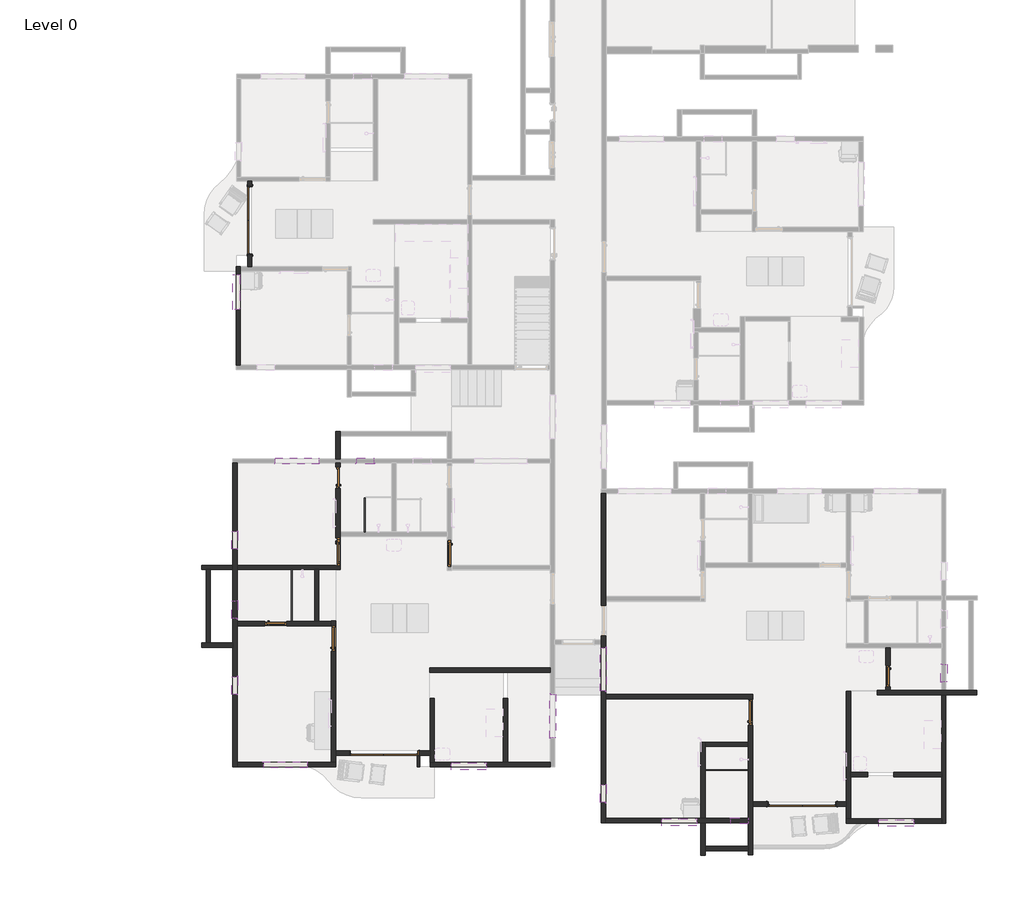
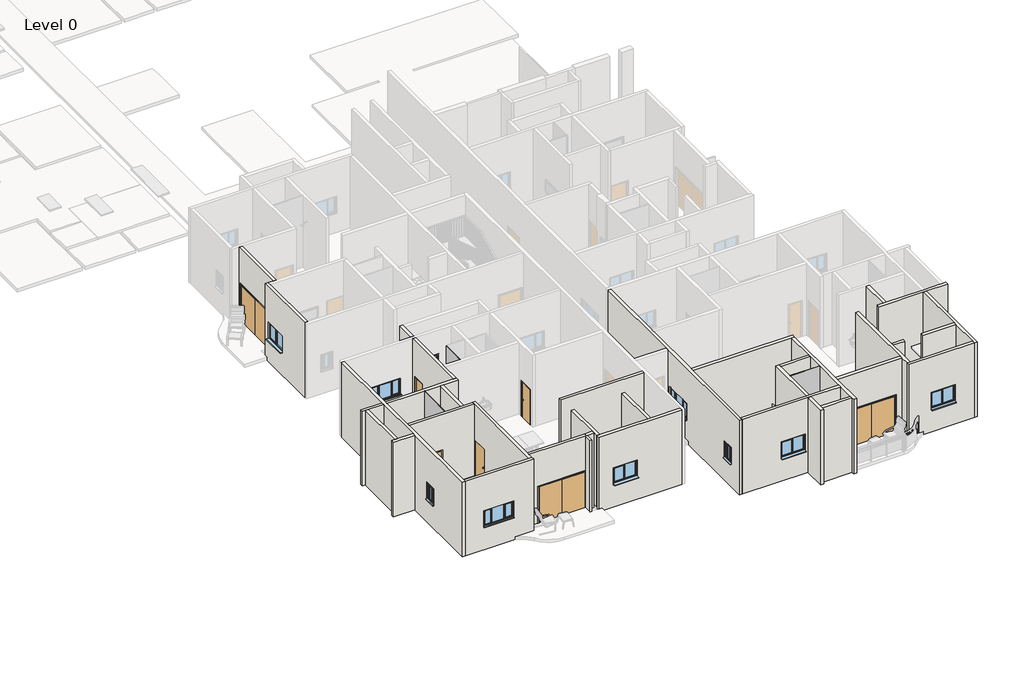
# One storey, part 1 of 14: 33 walls, 15 windows, 11 doors, 3 plates.
# Revit data of these elements (continued)
# Type "Windows_Tpl_Variable_Casement : 5'" (continued)
#   Visual Light Transmittance = 0.9
#   Solar Heat Gain Coefficient = 0.78
#   Rough Width = 1524 mm
#   Rough Height = 910 mm
#   Height = 910 mm
#   Width = 1524 mm
#   Heat Transfer Coefficient (U) = 3.6886 W/(m²·K)
#   Glazing Thickness = 24 mm
#   FrameOffset - External = 50 mm
#   Frame Depth = 65 mm
#   Default Head Height = 2110 mm
#   Cill Depth = 87.5 mm
#   Cavity Closer Width = 50 mm
#   Cavity Closer Offset from Ext = 102.5 mm
#   Cavity Closer Depth = 85 mm
#   Casement Width = 450 mm
#   Vis - Cavity Closers = yes
#   Define Thermal Properties by = 1
#   Material Trim = Window Frame
#   Material Glass = Glass
#   Material Frame = Window Frame
#   Wall Closure = (empty or 0)
# Elements 1, 2, 3 (IfcDoor, "Doors_Concept_IntDbl : 8'")
#   Phase Created = New Construction
#   Materials on its faces: "Glass", "Glass, Clear Glazing"
# Elements 4, 5, 6, 7, 8 (IfcDoor, "Doors_ExtSgl_Flush : D2")
#   Phase Created = New Construction
#   Materials on its faces: "Door - Handle", "Door - Frame/Mullion", "Door - Panel"
# Elements 9, 10, 11 (IfcDoor, "Doors_ExtSgl_Flush : D3")
#   Phase Created = New Construction
#   Materials on its faces: "Door - Handle", "Door - Frame/Mullion", "Door - Panel"
# Elements 12, 13, 14 (IfcPlate, "System Panel : Glazed")
#   Phase Created = New Construction
#   Materials on its faces: "Glass"
# Elements 15, 16, 17, 18, 19, 20, 21, 22, 23, 24, 25, 26, 27, 28, 29, 30, 31, 32, 33, 34, 35, 36, 37, 38, 39, 40, 41, 42, 43, 44, 45, 46 (IfcWall, "W1")
#   Top Offset = 0 mm
#   Base Offset = 0 mm
#   wall height = 4000 mm
#   Phase Created = New Construction
#   Base Constraint = Level 0
#   Top Constraint = Level 1
#   Materials on its faces: "Brick, Common"
# Element 47 (IfcWall, "W9")
#   Top Offset = 0 mm
#   Base Offset = 0 mm
#   wall height = 4000 mm
#   Phase Created = New Construction
#   Base Constraint = Level 0
#   Top Constraint = Level 1
#   Materials on its faces: "Brick, Common"
# Element 48 (IfcWindow, "Windows_Concept_Plain_Dbl : 4'")
#   Mark = "1"
#   Phase Created = New Construction
#   Materials on its faces: "Window Frame", "Glass"
# Element 49 (IfcWindow, "Windows_Concept_Plain_Dbl : 4'")
#   Mark = "12"
#   Phase Created = New Construction
#   Materials on its faces: "Window Frame", "Glass"
# Element 50 (IfcWindow, "Windows_Concept_Plain_Dbl : 4'")
#   Mark = "19"
#   Phase Created = New Construction
#   Materials on its faces: "Window Frame", "Glass"
# Element 51 (IfcWindow, "Windows_Concept_Plain_Dbl : 4'")
#   Mark = "65"
#   Phase Created = New Construction
#   Materials on its faces: "Window Frame", "Glass"
# Element 52 (IfcWindow, "Windows_Sgl_Plain : 2'")
#   Mark = "4"
#   Phase Created = New Construction
#   Materials on its faces: "Window Frame", "Glass"
# Element 53 (IfcWindow, "Windows_Sgl_Plain : 2'")
#   Mark = "5"
#   Phase Created = New Construction
#   Materials on its faces: "Window Frame", "Glass"
# Element 54 (IfcWindow, "Windows_Sgl_Plain : 2'")
#   Mark = "20"
#   Phase Created = New Construction
#   Materials on its faces: "Window Frame", "Glass"
# Element 55 (IfcWindow, "Windows_Sgl_Plain : 2'")
#   Mark = "23"
#   Phase Created = New Construction
#   Materials on its faces: "Window Frame", "Glass"
# Element 56 (IfcWindow, "Windows_Tpl_Variable_Casement : 2'")
#   Mark = "3"
#   Phase Created = New Construction
#   Materials on its faces: "Window Frame", "Glass"
# Element 57 (IfcWindow, "Windows_Tpl_Variable_Casement : 2'")
#   Mark = "7"
#   Phase Created = New Construction
#   Materials on its faces: "Window Frame", "Glass"
# Element 58 (IfcWindow, "Windows_Tpl_Variable_Casement : 2'")
#   Mark = "13"
#   Phase Created = New Construction
#   Materials on its faces: "Window Frame", "Glass"
# Element 59 (IfcWindow, "Windows_Tpl_Variable_Casement : 5'")
#   Mark = "2"
#   Phase Created = New Construction
#   Materials on its faces: "Window Frame", "Glass"
# Element 60 (IfcWindow, "Windows_Tpl_Variable_Casement : 5'")
#   Mark = "8"
#   Phase Created = New Construction
#   Materials on its faces: "Window Frame", "Glass"
# Element 61 (IfcWindow, "Windows_Tpl_Variable_Casement : 5'")
#   Mark = "10"
#   Phase Created = New Construction
#   Materials on its faces: "Window Frame", "Glass"
# Element 62 (IfcWindow, "Windows_Tpl_Variable_Casement : 5'")
#   Mark = "14"
#   Phase Created = New Construction
#   Materials on its faces: "Window Frame", "Glass"
# Materials
#   "Glass": class "Glass", colour RGB 0 128 192, transparency 0.9, Description = "Soda Lime Glass", Cost = 0
#   "Glass, Clear Glazing": class "Glass", colour RGB 0 128 192, transparency 0.75, Description = "Clear glazing", Cost = 0
#   "Door - Panel": class "Wood", colour RGB 210 159 95, transparency 0, Keynote = "L20", Cost = 0
#   "Door - Frame/Mullion": class "Wood", colour RGB 212 179 113, transparency 0, Keynote = "L20", Cost = 0
#   "Door - Handle": colour RGB 0 0 0, transparency 0, Keynote = "P21", Cost = 0
#   "Brick, Common": class "Masonry", colour RGB 170 100 105, transparency 0, Description = "Common brick", Cost = 0
#   "Window Frame": colour RGB 249 249 249, transparency 0, Keynote = "L10", Cost = 0
